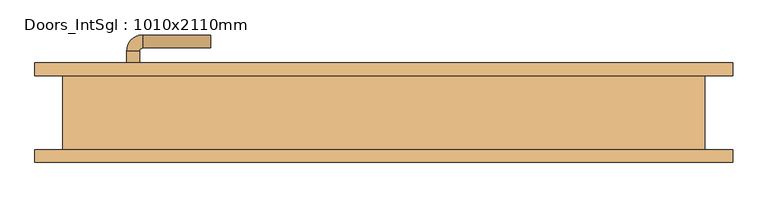
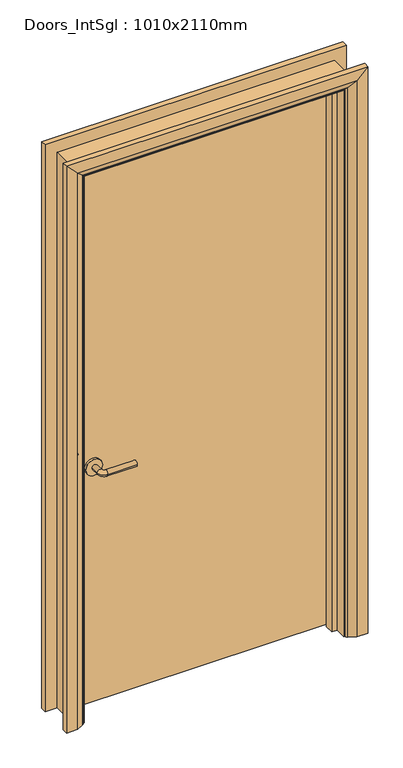
"""IFC4 building model written with IfcOpenShell, lengths in millimetres: door geometry, Doors_IntSgl : 1010x2110mm."""

from ifc_helpers import new_model, si_unit, point, frame, frame_2d, origin, place, context, project, spatial, polyline, circle_curve, ellipse_curve, trimmed, segment, composite_curve, outline, extrude, faceted_brep, source, transform, mapped, element, save
from ifc_brep_helpers import plane_surface, cylinder_surface, revolved_surface, advanced_brep


def doors_intsgl_1010x2110mm_a785dbed(model_context):
    return source(origin(), model_context, "Body", "SolidModel", [
        advanced_brep(
        [(-398.0, 11.15, 900.0), (-378.0, 11.15, 900.0), (-378.0, -18.85, 900.0), (-398.0, -18.85, 900.0), (-373.0, -23.85, 900.0), (-373.0, -43.85, 900.0), (-268.0, -43.85, 900.0), (-268.0, -23.85, 900.0)],
        [
            (0, 1, circle_curve(frame((-388.0, 11.15, 900.0), z_axis=(0.0, 1.0, 0.0), x_axis=(1.0, 0.0, 0.0)), 10.0)),
            (1, 0, circle_curve(frame((-388.0, 11.15, 900.0), z_axis=(0.0, 1.0, 0.0), x_axis=(1.0, 0.0, 0.0)), 10.0)),
            (1, 2),
            (2, 3, circle_curve(frame((-388.0, -18.85, 900.0), z_axis=(0.0, 1.0, 0.0), x_axis=(1.0, 0.0, 0.0)), 10.0)),
            (3, 0),
            (3, 2, circle_curve(frame((-388.0, -18.85, 900.0), z_axis=(0.0, 1.0, 0.0), x_axis=(1.0, 0.0, 0.0)), 10.0)),
            (4, 5, circle_curve(frame((-373.0, -33.85, 900.0), z_axis=(-1.0, 0.0, 0.0), x_axis=(0.0, 1.0, 0.0)), 10.0)),
            (5, 3, circle_curve(frame((-373.0, -18.85, 900.0), z_axis=(0.0, 0.0, -1.0), x_axis=(-1.0, 0.0, 0.0)), 25.0)),
            (2, 4, circle_curve(frame((-373.0, -18.85, 900.0), z_axis=(0.0, 0.0, 1.0), x_axis=(-1.0, 0.0, 0.0)), 5.0)),
            (5, 4, circle_curve(frame((-373.0, -33.85, 900.0), z_axis=(-1.0, 0.0, 0.0), x_axis=(0.0, 1.0, 0.0)), 10.0)),
            (6, 7, circle_curve(frame((-268.0, -33.85, 900.0), z_axis=(1.0, 0.0, 0.0), x_axis=(0.0, 1.0, 0.0)), 10.0)),
            (7, 6, circle_curve(frame((-268.0, -33.85, 900.0), z_axis=(1.0, 0.0, 0.0), x_axis=(0.0, 1.0, 0.0)), 10.0)),
            (4, 7),
            (6, 5),
        ],
        [
            plane_surface(frame((-388.0, 11.15, 900.0), z_axis=(0.0, 1.0, 0.0), x_axis=(0.0, 0.0, 1.0))),
            cylinder_surface(frame((-388.0, 11.15, 900.0), z_axis=(0.0, 1.0, 0.0), x_axis=(1.0, 0.0, 0.0)), 10.0),
            revolved_surface(trimmed(ellipse_curve(frame((-388.0, -18.85, 900.0), z_axis=(0.0, -1.0, 0.0), x_axis=(1.0, 0.0, 0.0)), 10.0, 10.0), [point((-398.0, -18.85, 900.0))], [point((-378.0, -18.85, 900.0))], True, "CARTESIAN"), (-373.0, -18.85, 900.0), (0.0, 0.0, -1.0)),
            revolved_surface(trimmed(ellipse_curve(frame((-388.0, -18.85, 900.0), z_axis=(0.0, -1.0, 0.0), x_axis=(1.0, 0.0, 0.0)), 10.0, 10.0), [point((-378.0, -18.85, 900.0))], [point((-398.0, -18.85, 900.0))], True, "CARTESIAN"), (-373.0, -18.85, 900.0), (0.0, 0.0, -1.0)),
            plane_surface(frame((-268.0, -33.85, 900.0), z_axis=(1.0, 0.0, 0.0), x_axis=(0.0, 0.0, 1.0))),
            cylinder_surface(frame((-373.0, -33.85, 900.0), z_axis=(-1.0, 0.0, 0.0), x_axis=(0.0, 1.0, 0.0)), 10.0),
        ],
        [
            (0, [[1, 2]]),
            (1, [[3, 4, 5, -2]]),
            (1, [[-5, 6, -3, -1]]),
            (2, [[7, 8, -4, 9]]),
            (3, [[10, -9, -6, -8]]),
            (4, [[11, 12]]),
            (5, [[13, -11, 14, -7]]),
            (5, [[-14, -12, -13, -10]]),
        ],
    ),
        extrude(outline(composite_curve([segment(trimmed(circle_curve(frame_2d((900.0, -390.5)), 30.0), [point((900.0, -420.5))], [point((900.0, -360.5))], False, "CARTESIAN"), True, "CONTINUOUS"), segment(trimmed(circle_curve(frame_2d((900.0, -390.5)), 30.0), [point((900.0, -360.5))], [point((900.0, -420.5))], False, "CARTESIAN"), True, "CONTINUOUS")], self_intersect=False)), frame((0.0, 11.15, 0.0), z_axis=(0.0, 1.0, 0.0), x_axis=(0.0, 0.0, 1.0)), (0.0, 0.0, 1.0), 8.0),
        advanced_brep(
        [(-398.0, 65.15, 900.0), (-378.0, 65.15, 900.0), (-398.0, 95.15, 900.0), (-378.0, 95.15, 900.0), (-373.0, 100.15, 900.0), (-373.0, 120.15, 900.0), (-268.0, 120.15, 900.0), (-268.0, 100.15, 900.0)],
        [
            (0, 1, circle_curve(frame((-388.0, 65.15, 900.0), z_axis=(0.0, -1.0, 0.0), x_axis=(1.0, 0.0, 0.0)), 10.0)),
            (1, 0, circle_curve(frame((-388.0, 65.15, 900.0), z_axis=(0.0, -1.0, 0.0), x_axis=(1.0, 0.0, 0.0)), 10.0)),
            (0, 2),
            (2, 3, circle_curve(frame((-388.0, 95.15, 900.0), z_axis=(0.0, -1.0, 0.0), x_axis=(1.0, 0.0, 0.0)), 10.0)),
            (3, 1),
            (3, 2, circle_curve(frame((-388.0, 95.15, 900.0), z_axis=(0.0, -1.0, 0.0), x_axis=(1.0, 0.0, 0.0)), 10.0)),
            (4, 3, circle_curve(frame((-373.0, 95.15, 900.0), z_axis=(0.0, 0.0, 1.0), x_axis=(-1.0, 0.0, 0.0)), 5.0)),
            (2, 5, circle_curve(frame((-373.0, 95.15, 900.0), z_axis=(0.0, 0.0, -1.0), x_axis=(-1.0, 0.0, 0.0)), 25.0)),
            (5, 4, circle_curve(frame((-373.0, 110.15, 900.0), z_axis=(-1.0, 0.0, 0.0), x_axis=(0.0, -1.0, 0.0)), 10.0)),
            (4, 5, circle_curve(frame((-373.0, 110.15, 900.0), z_axis=(-1.0, 0.0, 0.0), x_axis=(0.0, -1.0, 0.0)), 10.0)),
            (6, 7, circle_curve(frame((-268.0, 110.15, 900.0), z_axis=(1.0, 0.0, 0.0), x_axis=(0.0, -1.0, 0.0)), 10.0)),
            (7, 6, circle_curve(frame((-268.0, 110.15, 900.0), z_axis=(1.0, 0.0, 0.0), x_axis=(0.0, -1.0, 0.0)), 10.0)),
            (5, 6),
            (7, 4),
        ],
        [
            plane_surface(frame((-388.0, 65.15, 900.0), z_axis=(0.0, -1.0, 0.0), x_axis=(0.0, 0.0, 1.0))),
            cylinder_surface(frame((-388.0, 65.15, 900.0), z_axis=(0.0, -1.0, 0.0), x_axis=(1.0, 0.0, 0.0)), 10.0),
            revolved_surface(trimmed(ellipse_curve(frame((-388.0, 95.15, 900.0), z_axis=(0.0, -1.0, 0.0), x_axis=(1.0, 0.0, 0.0)), 10.0, 10.0), [point((-398.0, 95.15, 900.0))], [point((-378.0, 95.15, 900.0))], True, "CARTESIAN"), (-373.0, 95.15, 900.0), (0.0, 0.0, -1.0)),
            revolved_surface(trimmed(ellipse_curve(frame((-388.0, 95.15, 900.0), z_axis=(0.0, -1.0, 0.0), x_axis=(1.0, 0.0, 0.0)), 10.0, 10.0), [point((-378.0, 95.15, 900.0))], [point((-398.0, 95.15, 900.0))], True, "CARTESIAN"), (-373.0, 95.15, 900.0), (0.0, 0.0, -1.0)),
            plane_surface(frame((-268.0, 110.15, 900.0), z_axis=(1.0, 0.0, 0.0), x_axis=(0.0, 0.0, 1.0))),
            cylinder_surface(frame((-373.0, 110.15, 900.0), z_axis=(-1.0, 0.0, 0.0), x_axis=(0.0, -1.0, 0.0)), 10.0),
        ],
        [
            (0, [[1, 2]]),
            (1, [[-1, 3, 4, 5]]),
            (1, [[-2, -5, 6, -3]]),
            (2, [[7, -4, 8, 9]]),
            (3, [[-8, -6, -7, 10]]),
            (4, [[11, 12]]),
            (5, [[-9, 13, -12, 14]]),
            (5, [[-10, -14, -11, -13]]),
        ],
    ),
        extrude(outline(composite_curve([segment(trimmed(circle_curve(frame_2d((900.0, -390.5)), 30.0), [point((900.0, -420.5))], [point((900.0, -360.5))], False, "CARTESIAN"), True, "CONTINUOUS"), segment(trimmed(circle_curve(frame_2d((900.0, -390.5)), 30.0), [point((900.0, -360.5))], [point((900.0, -420.5))], False, "CARTESIAN"), True, "CONTINUOUS")], self_intersect=False)), frame((0.0, 57.15, 0.0), z_axis=(0.0, 1.0, 0.0), x_axis=(0.0, 0.0, 1.0)), (0.0, 0.0, 1.0), 8.0),
        extrude(outline(polyline([(463.0, 19.15), (-463.0, 19.15), (-463.0, 57.15), (463.0, 57.15), (463.0, 19.15)])), frame((0.0, 0.0, 8.0), z_axis=(0.0, 0.0, 1.0), x_axis=(1.0, 0.0, 0.0)), (0.0, 0.0, 1.0), 2060.0),
        advanced_brep(
        [(540.0, 77.15, 0.0), (540.0, 57.15, 0.0), (470.0, 57.15, 0.0), (474.0, 63.15, 0.0), (500.0, 77.15, 0.0), (540.0, 77.15, 2145.0), (540.0, 57.15, 2145.0), (-540.0, 57.15, 2145.0), (-540.0, 57.15, 0.0), (-470.0, 57.15, 0.0), (-470.0, 57.15, 2075.0), (470.0, 57.15, 2075.0), (474.0, 63.15, 2079.0), (500.0, 77.15, 2105.0), (-500.0, 77.15, 2105.0), (-500.0, 77.15, 0.0), (-540.0, 77.15, 0.0), (-540.0, 77.15, 2145.0), (-474.0, 63.15, 2079.0), (-474.0, 63.15, 0.0)],
        [
            (0, 1),
            (1, 2),
            (2, 3, circle_curve(frame((478.0, 56.15, 0.0), z_axis=(0.0, 0.0, -1.0), x_axis=(1.0, 0.0, 0.0)), 8.0622577)),
            (3, 4),
            (4, 0),
            (0, 5),
            (5, 6),
            (6, 1),
            (6, 7),
            (7, 8),
            (8, 9),
            (9, 10),
            (10, 11),
            (11, 2),
            (11, 12, ellipse_curve(frame((478.0, 56.15, 2083.0), z_axis=(0.7071067811865475, 0.0, -0.7071067811865475), x_axis=(-0.7071067811865474, 0.0, -0.7071067811865476)), 11.4017543, 8.0622577)),
            (12, 3),
            (12, 13),
            (13, 4),
            (13, 14),
            (14, 15),
            (15, 16),
            (16, 17),
            (17, 5),
            (17, 7),
            (10, 18, ellipse_curve(frame((-478.0, 56.15, 2083.0), z_axis=(0.7071067811865475, 0.0, 0.7071067811865475), x_axis=(0.7071067811865476, 0.0, -0.7071067811865474)), 11.4017543, 8.0622577)),
            (18, 12),
            (18, 14),
            (15, 19),
            (19, 9, circle_curve(frame((-478.0, 56.15, 0.0), z_axis=(0.0, 0.0, -1.0), x_axis=(-1.0, 0.0, 0.0)), 8.0622577)),
            (8, 16),
            (19, 18),
        ],
        [
            plane_surface(frame((470.0, 57.15, 0.0), z_axis=(0.0, 0.0, -1.0), x_axis=(0.0, -1.0, 0.0))),
            plane_surface(frame((540.0, 77.15, 0.0), z_axis=(1.0, 0.0, 0.0), x_axis=(0.0, 0.0, 1.0))),
            plane_surface(frame((540.0, 57.15, 0.0), z_axis=(0.0, -1.0, 0.0), x_axis=(0.0, 0.0, 1.0))),
            cylinder_surface(frame((478.0, 56.15, 0.0), z_axis=(0.0, 0.0, -1.0), x_axis=(1.0, 0.0, 0.0)), 8.0622577),
            plane_surface(frame((474.0, 63.15, 0.0), z_axis=(-0.4740998230350126, 0.880471099922178, 0.0), x_axis=(0.0, 0.0, 1.0))),
            plane_surface(frame((500.0, 77.15, 0.0), z_axis=(0.0, 1.0, 0.0), x_axis=(0.0, 0.0, 1.0))),
            plane_surface(frame((540.0, 77.15, 2145.0), z_axis=(0.0, 0.0, 1.0), x_axis=(-1.0, 0.0, 0.0))),
            cylinder_surface(frame((470.0, 56.15, 2083.0), z_axis=(1.0, 0.0, 0.0), x_axis=(0.0, 0.0, 1.0)), 8.0622577),
            plane_surface(frame((474.0, 63.15, 2079.0), z_axis=(0.0, 0.8804710999221764, -0.4740998230350154), x_axis=(-1.0, 0.0, 0.0))),
            plane_surface(frame((-470.0, 57.15, 0.0), z_axis=(0.0, 0.0, -1.0), x_axis=(0.0, -1.0, 0.0))),
            plane_surface(frame((-540.0, 77.15, 2145.0), z_axis=(-1.0, 0.0, 0.0), x_axis=(0.0, 0.0, -1.0))),
            cylinder_surface(frame((-478.0, 56.15, 2075.0), z_axis=(0.0, 0.0, 1.0), x_axis=(-1.0, 0.0, 0.0)), 8.0622577),
            plane_surface(frame((-474.0, 63.15, 2079.0), z_axis=(0.47409982303501824, 0.8804710999221749, 0.0), x_axis=(0.0, 0.0, -1.0))),
        ],
        [
            (0, [[1, 2, 3, 4, 5]]),
            (1, [[-1, 6, 7, 8]]),
            (2, [[-2, -8, 9, 10, 11, 12, 13, 14]]),
            (3, [[-3, -14, 15, 16]]),
            (4, [[-4, -16, 17, 18]]),
            (5, [[-5, -18, 19, 20, 21, 22, 23, -6]]),
            (6, [[-7, -23, 24, -9]]),
            (7, [[-15, -13, 25, 26]]),
            (8, [[-17, -26, 27, -19]]),
            (9, [[-21, 28, 29, -11, 30]]),
            (10, [[-24, -22, -30, -10]]),
            (11, [[-25, -12, -29, 31]]),
            (12, [[-27, -31, -28, -20]]),
        ],
    ),
        extrude(outline(polyline([(0.0, -465.0), (0.0, -446.0), (2051.0, -446.0), (2051.0, 446.0), (0.0, 446.0), (0.0, 465.0), (2070.0, 465.0), (2070.0, -465.0), (0.0, -465.0)])), frame((0.0, -14.85, 0.0), z_axis=(0.0, 1.0, 0.0), x_axis=(0.0, 0.0, 1.0)), (0.0, 0.0, 1.0), 32.0),
        advanced_brep(
        [(-540.0, -77.15, 0.0), (-540.0, -57.15, 0.0), (-470.0, -57.15, 0.0), (-474.0, -63.15, 0.0), (-500.0, -77.15, 0.0), (-540.0, -77.15, 2145.0), (-540.0, -57.15, 2145.0), (-470.0, -57.15, 2075.0), (-474.0, -63.15, 2079.0), (-500.0, -77.15, 2105.0), (540.0, -77.15, 2145.0), (540.0, -57.15, 2145.0), (470.0, -57.15, 2075.0), (474.0, -63.15, 2079.0), (500.0, -77.15, 2105.0), (540.0, -77.15, 0.0), (500.0, -77.15, 0.0), (474.0, -63.15, 0.0), (470.0, -57.15, 0.0), (540.0, -57.15, 0.0)],
        [
            (0, 1),
            (1, 2),
            (2, 3, circle_curve(frame((-478.0, -56.15, 0.0), z_axis=(0.0, 0.0, -1.0), x_axis=(-1.0, 0.0, 0.0)), 8.0622577)),
            (3, 4),
            (4, 0),
            (0, 5),
            (5, 6),
            (6, 1),
            (6, 7),
            (7, 2),
            (7, 8, ellipse_curve(frame((-478.0, -56.15, 2083.0), z_axis=(-0.7071067811865475, 0.0, -0.7071067811865475), x_axis=(0.7071067811865474, 0.0, -0.7071067811865476)), 11.4017543, 8.0622577)),
            (8, 3),
            (8, 9),
            (9, 4),
            (9, 5),
            (5, 10),
            (10, 11),
            (11, 6),
            (11, 12),
            (12, 7),
            (12, 13, ellipse_curve(frame((478.0, -56.15, 2083.0), z_axis=(-0.7071067811865475, 0.0, 0.7071067811865475), x_axis=(-0.7071067811865476, 0.0, -0.7071067811865474)), 11.4017543, 8.0622577)),
            (13, 8),
            (13, 14),
            (14, 9),
            (14, 10),
            (15, 16),
            (16, 17),
            (17, 18, circle_curve(frame((478.0, -56.15, 0.0), z_axis=(0.0, 0.0, -1.0), x_axis=(1.0, 0.0, 0.0)), 8.0622577)),
            (18, 19),
            (19, 15),
            (10, 15),
            (19, 11),
            (18, 12),
            (17, 13),
            (16, 14),
        ],
        [
            plane_surface(frame((-470.0, -129.9510989, 0.0), z_axis=(0.0, 0.0, -1.0), x_axis=(1.0, 0.0, 0.0))),
            plane_surface(frame((-540.0, -77.15, 0.0), z_axis=(-1.0, 0.0, 0.0), x_axis=(0.0, 0.0, 1.0))),
            plane_surface(frame((-540.0, -57.15, 0.0), z_axis=(0.0, 1.0, 0.0), x_axis=(0.0, 0.0, 1.0))),
            cylinder_surface(frame((-478.0, -56.15, 0.0), z_axis=(0.0, 0.0, -1.0), x_axis=(-1.0, 0.0, 0.0)), 8.0622577),
            plane_surface(frame((-474.0, -63.15, 0.0), z_axis=(0.4740998230350183, -0.8804710999221749, 0.0), x_axis=(0.0, 0.0, 1.0))),
            plane_surface(frame((-500.0, -77.15, 0.0), z_axis=(0.0, -1.0, 0.0), x_axis=(0.0, 0.0, 1.0))),
            plane_surface(frame((-540.0, -77.15, 2145.0), z_axis=(0.0, 0.0, 1.0), x_axis=(1.0, 0.0, 0.0))),
            plane_surface(frame((-540.0, -57.15, 2145.0), z_axis=(0.0, 1.0, 0.0), x_axis=(1.0, 0.0, 0.0))),
            cylinder_surface(frame((-470.0, -56.15, 2083.0), z_axis=(-1.0, 0.0, 0.0), x_axis=(0.0, 0.0, 1.0)), 8.0622577),
            plane_surface(frame((-474.0, -63.15, 2079.0), z_axis=(0.0, -0.8804710999221749, -0.4740998230350183), x_axis=(1.0, 0.0, 0.0))),
            plane_surface(frame((-500.0, -77.15, 2105.0), z_axis=(0.0, -1.0, 0.0), x_axis=(1.0, 0.0, 0.0))),
            plane_surface(frame((470.0, -129.9510989, 0.0), z_axis=(0.0, 0.0, -1.0), x_axis=(-1.0, 0.0, 0.0))),
            plane_surface(frame((540.0, -77.15, 2145.0), z_axis=(1.0, 0.0, 0.0), x_axis=(0.0, 0.0, -1.0))),
            plane_surface(frame((540.0, -57.15, 2145.0), z_axis=(0.0, 1.0, 0.0), x_axis=(0.0, 0.0, -1.0))),
            cylinder_surface(frame((478.0, -56.15, 2075.0), z_axis=(0.0, 0.0, 1.0), x_axis=(1.0, 0.0, 0.0)), 8.0622577),
            plane_surface(frame((474.0, -63.15, 2079.0), z_axis=(-0.4740998230350183, -0.8804710999221749, 0.0), x_axis=(0.0, 0.0, -1.0))),
            plane_surface(frame((500.0, -77.15, 2105.0), z_axis=(0.0, -1.0, 0.0), x_axis=(0.0, 0.0, -1.0))),
        ],
        [
            (0, [[1, 2, 3, 4, 5]]),
            (1, [[-1, 6, 7, 8]]),
            (2, [[-2, -8, 9, 10]]),
            (3, [[-3, -10, 11, 12]]),
            (4, [[-4, -12, 13, 14]]),
            (5, [[-5, -14, 15, -6]]),
            (6, [[-7, 16, 17, 18]]),
            (7, [[-9, -18, 19, 20]]),
            (8, [[-11, -20, 21, 22]]),
            (9, [[-13, -22, 23, 24]]),
            (10, [[-15, -24, 25, -16]]),
            (11, [[26, 27, 28, 29, 30]]),
            (12, [[-17, 31, -30, 32]]),
            (13, [[-19, -32, -29, 33]]),
            (14, [[-21, -33, -28, 34]]),
            (15, [[-23, -34, -27, 35]]),
            (16, [[-25, -35, -26, -31]]),
        ],
    ),
        faceted_brep([(-465.0, 57.15, 0.0), (-465.0, -57.15, 0.0), (-497.0, -57.15, 0.0), (-497.0, 57.15, 0.0), (-465.0, 57.15, 2070.0), (-465.0, -57.15, 2070.0), (-497.0, -57.15, 2102.0), (-497.0, 57.15, 2102.0), (465.0, 57.15, 2070.0), (465.0, -57.15, 2070.0), (497.0, -57.15, 2102.0), (497.0, 57.15, 2102.0), (465.0, 57.15, 0.0), (497.0, 57.15, 0.0), (497.0, -57.15, 0.0), (465.0, -57.15, 0.0)], [[[0, 1, 2, 3]], [[1, 0, 4, 5]], [[2, 1, 5, 6]], [[3, 2, 6, 7]], [[0, 3, 7, 4]], [[5, 4, 8, 9]], [[6, 5, 9, 10]], [[7, 6, 10, 11]], [[4, 7, 11, 8]], [[12, 13, 14, 15]], [[9, 8, 12, 15]], [[10, 9, 15, 14]], [[11, 10, 14, 13]], [[8, 11, 13, 12]]]),
    ])


if __name__ == "__main__":
    model = new_model("IFC4")
    model_context = context("Model", 3, world=origin())
    ifc_project = project(units=[si_unit("LENGTHUNIT", "METRE", prefix="MILLI")], contexts=[model_context])
    site = spatial("IfcSite", under=ifc_project)
    building = spatial("IfcBuilding", under=site)
    placement = place(None, origin())
    doors_intsgl_1010x2110mm_shape = doors_intsgl_1010x2110mm_a785dbed(model_context)
    element("IfcDoor", 1, ObjectType="Doors_IntSgl : 1010x2110mm", at=placement, inside=building, context=model_context, shape_type="MappedRepresentation", body=[
        mapped(doors_intsgl_1010x2110mm_shape, transform((0.0, 0.0, 0.0), x_axis=(1.0, 0.0, 0.0), y_axis=(0.0, 1.0, 0.0), z_axis=(0.0, 0.0, 1.0))),
    ])
    save(model, "model.ifc")

# Revit data of these elements
# Type "Doors_IntSgl : 1010x2110mm"
#   Construction Type Id = "MDOOR"
#   Type Mark = "43"
#   Type Comments = "Internal Single"
#   Operation = "SingleSwingRight"
#   Manufacturer = "Revit"
#   Keynote = "L20"
#   Description = "Internal Single Door"
#   Analytic Construction = "Metal"
#   UnderCut = 8 mm
#   Tolerance = 2 mm
#   Thickness = 38 mm
#   Thermal Resistance (R) = 0.270117 (m²·K)/W
#   Structural Tolerance = 8 mm
#   StopDepth = 32 mm
#   Stop Thickness = 19 mm
#   Rough Width = 1010 mm
#   Rough Height = 2110 mm
#   Height to Top Lock Rail = 1000 mm
#   Heat Transfer Coefficient (U) = 3.7021 W/(m²·K)
#   Handle Z Distance = 900 mm
#   Handle X Distance = 75 mm
#   Frame Thickness = 32 mm
#   Door Panel Width = 926 mm
#   Door Panel Thickness = 38 mm
#   Door Panel Offset = 0 mm
#   Height = 2110 mm
#   Width = 1010 mm
#   Door Panel Height = 2060 mm
#   Architrave Setback = 5 mm
#   Define Thermal Properties by = 1
#   Vis - Ironmongery = yes
#   Material Ironmongery = Door - Handle
#   Material Frame = Door - Frame/Mullion (1)
#   Material Door = Door - Panel
#   Material Architrave = Door - Architrave
#   Visual Light Transmittance = 0
#   Solar Heat Gain Coefficient = 0
#   Function = (empty or 0)
#   Wall Closure = (empty or 0)
# Element 1 (IfcDoor, "Doors_IntSgl : 1010x2110mm")
#   Materials on its faces: "Door - Architrave", "Door - Handle", "Door - Frame/Mullion (1)", "Door - Panel"
# Materials
#   "Door - Handle": colour RGB 0 0 0, transparency 0, Keynote = "P21", Cost = 0
#   "Door - Frame/Mullion (1)": class "Wood", colour RGB 212 179 113, transparency 0, Keynote = "L20", Cost = 0
#   "Door - Panel": class "Wood", colour RGB 210 159 95, transparency 0, Keynote = "L20", Cost = 0
#   "Door - Architrave": class "Wood", colour RGB 154 90 5, transparency 0, Keynote = "P20", Cost = 0
